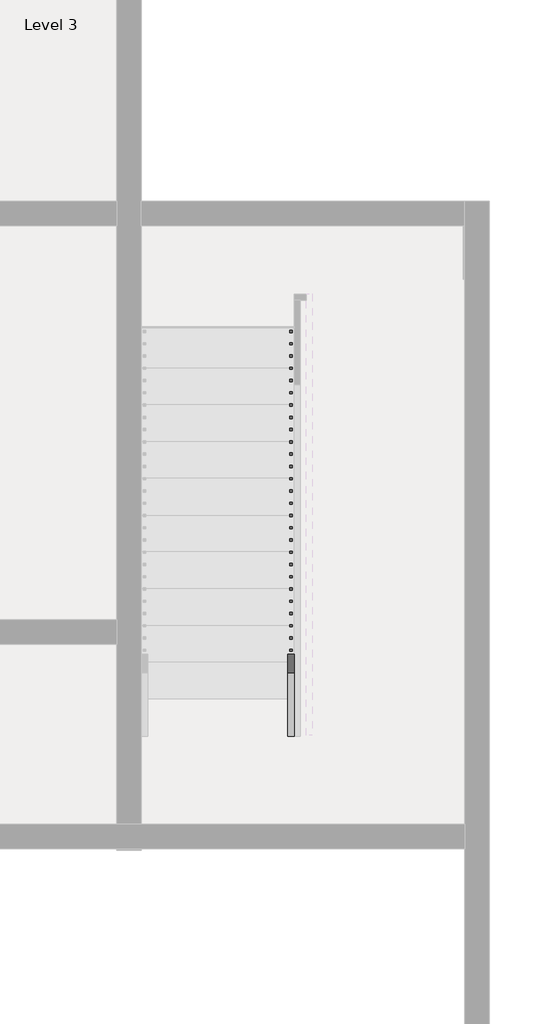
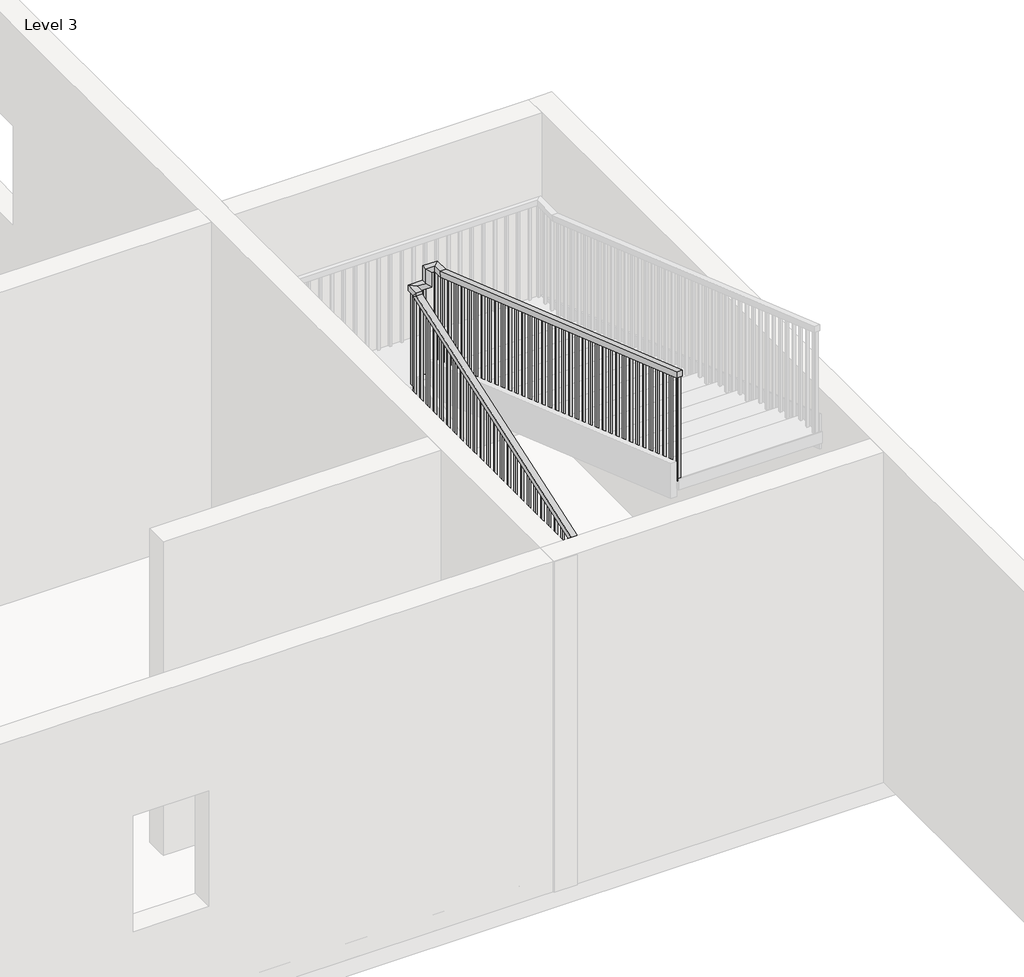
# One storey, part 6 of 14: 1 railing.
"""IFC4 building model written with IfcOpenShell, lengths in millimetres."""

from ifc_helpers import new_model, si_unit, frame, origin, place, context, project, spatial, polyline, outline, extrude, faceted_brep, element, save

model = new_model("IFC4")

# Units and contexts
model_context = context("Model", 3, world=origin())
ifc_project = project(units=[si_unit("LENGTHUNIT", "METRE", prefix="MILLI")], contexts=[model_context])

# Site, building, storey
site = spatial("IfcSite", under=ifc_project)
building = spatial("IfcBuilding", under=site)
storey = spatial("IfcBuildingStorey", under=building, Name="Level 3", Elevation=6096.0)

# Railing
placement = place(None, origin())
element("IfcRailing", 1, ObjectType="Handrail - Rectangular", at=placement, inside=storey, context=model_context, shape_type="SolidModel", body=[
    faceted_brep([(-2644.5381751, -9955.5916506, 7115.9076923), (-2644.5381751, -9955.5916506, 7062.1602476), (-2593.7381751, -9955.5916506, 7062.1602476), (-2593.7381751, -9955.5916506, 7115.9076923), (-2644.5381751, -6367.8416506, 8355.6687908), (-2644.5381751, -6317.0416506, 8319.4754856), (-2593.7381751, -6317.0416506, 8319.4754856), (-2593.7381751, -6367.8416506, 8355.6687908), (-2644.5381751, -6367.8416506, 8382.0), (-2644.5381751, -6317.0416506, 8331.2), (-2593.7381751, -6317.0416506, 8331.2), (-2593.7381751, -6367.8416506, 8382.0), (-2644.5381751, -6240.8416506, 8382.0), (-2644.5381751, -6240.8416506, 8331.2), (-2593.7381751, -6291.6416506, 8331.2), (-2593.7381751, -6291.6416506, 8382.0), (-2517.5381751, -6240.8416506, 8382.0), (-2466.7381751, -6240.8416506, 8331.2), (-2466.7381751, -6291.6416506, 8331.2), (-2517.5381751, -6291.6416506, 8382.0), (-2517.5381751, -6240.8416506, 8513.8846154), (-2466.7381751, -6240.8416506, 8463.0846154), (-2466.7381751, -6291.6416506, 8463.0846154), (-2517.5381751, -6291.6416506, 8513.8846154), (-2390.5381751, -6240.8416506, 8513.8846154), (-2390.5381751, -6240.8416506, 8463.0846154), (-2441.3381751, -6291.6416506, 8463.0846154), (-2441.3381751, -6291.6416506, 8513.8846154), (-2390.5381751, -6367.8416506, 8513.8846154), (-2390.5381751, -6376.3852679, 8463.0846154), (-2441.3381751, -6376.3852679, 8463.0846154), (-2441.3381751, -6367.8416506, 8513.8846154), (-2390.5381751, -9949.2416506, 9753.6), (-2441.3381751, -9949.2416506, 9753.6), (-2441.3381751, -9949.2416506, 9699.842594), (-2390.5381751, -9949.2416506, 9699.842594)], [[[0, 1, 2, 3]], [[1, 0, 4, 5]], [[2, 1, 5, 6]], [[3, 2, 6, 7]], [[0, 3, 7, 4]], [[5, 4, 8, 9]], [[6, 5, 9, 10]], [[7, 6, 10, 11]], [[4, 7, 11, 8]], [[9, 8, 12, 13]], [[10, 9, 13, 14]], [[11, 10, 14, 15]], [[8, 11, 15, 12]], [[13, 12, 16, 17]], [[14, 13, 17, 18]], [[15, 14, 18, 19]], [[12, 15, 19, 16]], [[17, 16, 20, 21]], [[18, 17, 21, 22]], [[19, 18, 22, 23]], [[16, 19, 23, 20]], [[21, 20, 24, 25]], [[22, 21, 25, 26]], [[23, 22, 26, 27]], [[20, 23, 27, 24]], [[25, 24, 28, 29]], [[26, 25, 29, 30]], [[27, 26, 30, 31]], [[24, 27, 31, 28]], [[32, 33, 34, 35]], [[29, 28, 32, 35]], [[30, 29, 35, 34]], [[31, 30, 34, 33]], [[28, 31, 33, 32]]]),
    extrude(outline(polyline([(-9933.3666506, 9694.3474017), (-9914.3166506, 9687.7531709), (-9914.3166506, 8733.6923077), (-9933.3666506, 8733.6923077), (-9933.3666506, 9694.3474017)])), frame((-2425.4631751, 0.0, 0.0), z_axis=(1.0, 0.0, 0.0), x_axis=(0.0, 1.0, 0.0)), (0.0, 0.0, 1.0), 19.05),
    extrude(outline(polyline([(-9831.7666506, 9659.1781709), (-9812.7166506, 9652.5839402), (-9812.7166506, 8733.6923077), (-9831.7666506, 8733.6923077), (-9831.7666506, 9659.1781709)])), frame((-2425.4631751, 0.0, 0.0), z_axis=(1.0, 0.0, 0.0), x_axis=(0.0, 1.0, 0.0)), (0.0, 0.0, 1.0), 19.05),
    extrude(outline(polyline([(-9730.1666506, 9624.0089402), (-9711.1166506, 9617.4147094), (-9711.1166506, 8733.6923077), (-9730.1666506, 8733.6923077), (-9730.1666506, 9624.0089402)])), frame((-2425.4631751, 0.0, 0.0), z_axis=(1.0, 0.0, 0.0), x_axis=(0.0, 1.0, 0.0)), (0.0, 0.0, 1.0), 19.05),
    extrude(outline(polyline([(-9628.5666506, 9588.8397094), (-9609.5166506, 9582.2454786), (-9609.5166506, 8628.1846154), (-9628.5666506, 8628.1846154), (-9628.5666506, 9588.8397094)])), frame((-2425.4631751, 0.0, 0.0), z_axis=(1.0, 0.0, 0.0), x_axis=(0.0, 1.0, 0.0)), (0.0, 0.0, 1.0), 19.05),
    extrude(outline(polyline([(-9526.9666506, 9553.6704786), (-9507.9166506, 9547.0762479), (-9507.9166506, 8628.1846154), (-9526.9666506, 8628.1846154), (-9526.9666506, 9553.6704786)])), frame((-2425.4631751, 0.0, 0.0), z_axis=(1.0, 0.0, 0.0), x_axis=(0.0, 1.0, 0.0)), (0.0, 0.0, 1.0), 19.05),
    extrude(outline(polyline([(-9425.3666506, 9518.5012479), (-9406.3166506, 9511.9070171), (-9406.3166506, 8628.1846154), (-9425.3666506, 8628.1846154), (-9425.3666506, 9518.5012479)])), frame((-2425.4631751, 0.0, 0.0), z_axis=(1.0, 0.0, 0.0), x_axis=(0.0, 1.0, 0.0)), (0.0, 0.0, 1.0), 19.05),
    extrude(outline(polyline([(-9323.7666506, 9483.3320171), (-9304.7166506, 9476.7377863), (-9304.7166506, 8522.6769231), (-9323.7666506, 8522.6769231), (-9323.7666506, 9483.3320171)])), frame((-2425.4631751, 0.0, 0.0), z_axis=(1.0, 0.0, 0.0), x_axis=(0.0, 1.0, 0.0)), (0.0, 0.0, 1.0), 19.05),
    extrude(outline(polyline([(-9222.1666506, 9448.1627863), (-9203.1166506, 9441.5685556), (-9203.1166506, 8522.6769231), (-9222.1666506, 8522.6769231), (-9222.1666506, 9448.1627863)])), frame((-2425.4631751, 0.0, 0.0), z_axis=(1.0, 0.0, 0.0), x_axis=(0.0, 1.0, 0.0)), (0.0, 0.0, 1.0), 19.05),
    extrude(outline(polyline([(-9120.5666506, 9412.9935556), (-9101.5166506, 9406.3993248), (-9101.5166506, 8522.6769231), (-9120.5666506, 8522.6769231), (-9120.5666506, 9412.9935556)])), frame((-2425.4631751, 0.0, 0.0), z_axis=(1.0, 0.0, 0.0), x_axis=(0.0, 1.0, 0.0)), (0.0, 0.0, 1.0), 19.05),
    extrude(outline(polyline([(-9018.9666506, 9377.8243248), (-8999.9166506, 9371.230094), (-8999.9166506, 8417.1692308), (-9018.9666506, 8417.1692308), (-9018.9666506, 9377.8243248)])), frame((-2425.4631751, 0.0, 0.0), z_axis=(1.0, 0.0, 0.0), x_axis=(0.0, 1.0, 0.0)), (0.0, 0.0, 1.0), 19.05),
    extrude(outline(polyline([(-8917.3666506, 9342.655094), (-8898.3166506, 9336.0608632), (-8898.3166506, 8417.1692308), (-8917.3666506, 8417.1692308), (-8917.3666506, 9342.655094)])), frame((-2425.4631751, 0.0, 0.0), z_axis=(1.0, 0.0, 0.0), x_axis=(0.0, 1.0, 0.0)), (0.0, 0.0, 1.0), 19.05),
    extrude(outline(polyline([(-8815.7666506, 9307.4858632), (-8796.7166506, 9300.8916325), (-8796.7166506, 8417.1692308), (-8815.7666506, 8417.1692308), (-8815.7666506, 9307.4858632)])), frame((-2425.4631751, 0.0, 0.0), z_axis=(1.0, 0.0, 0.0), x_axis=(0.0, 1.0, 0.0)), (0.0, 0.0, 1.0), 19.05),
    extrude(outline(polyline([(-8714.1666506, 9272.3166325), (-8695.1166506, 9265.7224017), (-8695.1166506, 8311.6615385), (-8714.1666506, 8311.6615385), (-8714.1666506, 9272.3166325)])), frame((-2425.4631751, 0.0, 0.0), z_axis=(1.0, 0.0, 0.0), x_axis=(0.0, 1.0, 0.0)), (0.0, 0.0, 1.0), 19.05),
    extrude(outline(polyline([(-8612.5666506, 9237.1474017), (-8593.5166506, 9230.5531709), (-8593.5166506, 8311.6615385), (-8612.5666506, 8311.6615385), (-8612.5666506, 9237.1474017)])), frame((-2425.4631751, 0.0, 0.0), z_axis=(1.0, 0.0, 0.0), x_axis=(0.0, 1.0, 0.0)), (0.0, 0.0, 1.0), 19.05),
    extrude(outline(polyline([(-8510.9666506, 9201.9781709), (-8491.9166506, 9195.3839402), (-8491.9166506, 8311.6615385), (-8510.9666506, 8311.6615385), (-8510.9666506, 9201.9781709)])), frame((-2425.4631751, 0.0, 0.0), z_axis=(1.0, 0.0, 0.0), x_axis=(0.0, 1.0, 0.0)), (0.0, 0.0, 1.0), 19.05),
    extrude(outline(polyline([(-8409.3666506, 9166.8089402), (-8390.3166506, 9160.2147094), (-8390.3166506, 8206.1538462), (-8409.3666506, 8206.1538462), (-8409.3666506, 9166.8089402)])), frame((-2425.4631751, 0.0, 0.0), z_axis=(1.0, 0.0, 0.0), x_axis=(0.0, 1.0, 0.0)), (0.0, 0.0, 1.0), 19.05),
    extrude(outline(polyline([(-8307.7666506, 9131.6397094), (-8288.7166506, 9125.0454786), (-8288.7166506, 8206.1538462), (-8307.7666506, 8206.1538462), (-8307.7666506, 9131.6397094)])), frame((-2425.4631751, 0.0, 0.0), z_axis=(1.0, 0.0, 0.0), x_axis=(0.0, 1.0, 0.0)), (0.0, 0.0, 1.0), 19.05),
    extrude(outline(polyline([(-8206.1666506, 9096.4704786), (-8187.1166506, 9089.8762479), (-8187.1166506, 8206.1538462), (-8206.1666506, 8206.1538462), (-8206.1666506, 9096.4704786)])), frame((-2425.4631751, 0.0, 0.0), z_axis=(1.0, 0.0, 0.0), x_axis=(0.0, 1.0, 0.0)), (0.0, 0.0, 1.0), 19.05),
    extrude(outline(polyline([(-8104.5666506, 9061.3012479), (-8085.5166506, 9054.7070171), (-8085.5166506, 8100.6461538), (-8104.5666506, 8100.6461538), (-8104.5666506, 9061.3012479)])), frame((-2425.4631751, 0.0, 0.0), z_axis=(1.0, 0.0, 0.0), x_axis=(0.0, 1.0, 0.0)), (0.0, 0.0, 1.0), 19.05),
    extrude(outline(polyline([(-8002.9666506, 9026.1320171), (-7983.9166506, 9019.5377863), (-7983.9166506, 8100.6461538), (-8002.9666506, 8100.6461538), (-8002.9666506, 9026.1320171)])), frame((-2425.4631751, 0.0, 0.0), z_axis=(1.0, 0.0, 0.0), x_axis=(0.0, 1.0, 0.0)), (0.0, 0.0, 1.0), 19.05),
    extrude(outline(polyline([(-7901.3666506, 8990.9627863), (-7882.3166506, 8984.3685556), (-7882.3166506, 8100.6461538), (-7901.3666506, 8100.6461538), (-7901.3666506, 8990.9627863)])), frame((-2425.4631751, 0.0, 0.0), z_axis=(1.0, 0.0, 0.0), x_axis=(0.0, 1.0, 0.0)), (0.0, 0.0, 1.0), 19.05),
    extrude(outline(polyline([(-7799.7666506, 8955.7935556), (-7780.7166506, 8949.1993248), (-7780.7166506, 7995.1384615), (-7799.7666506, 7995.1384615), (-7799.7666506, 8955.7935556)])), frame((-2425.4631751, 0.0, 0.0), z_axis=(1.0, 0.0, 0.0), x_axis=(0.0, 1.0, 0.0)), (0.0, 0.0, 1.0), 19.05),
    extrude(outline(polyline([(-7698.1666506, 8920.6243248), (-7679.1166506, 8914.030094), (-7679.1166506, 7995.1384615), (-7698.1666506, 7995.1384615), (-7698.1666506, 8920.6243248)])), frame((-2425.4631751, 0.0, 0.0), z_axis=(1.0, 0.0, 0.0), x_axis=(0.0, 1.0, 0.0)), (0.0, 0.0, 1.0), 19.05),
    extrude(outline(polyline([(-7596.5666506, 8885.455094), (-7577.5166506, 8878.8608632), (-7577.5166506, 7995.1384615), (-7596.5666506, 7995.1384615), (-7596.5666506, 8885.455094)])), frame((-2425.4631751, 0.0, 0.0), z_axis=(1.0, 0.0, 0.0), x_axis=(0.0, 1.0, 0.0)), (0.0, 0.0, 1.0), 19.05),
    extrude(outline(polyline([(-7494.9666506, 8850.2858632), (-7475.9166506, 8843.6916325), (-7475.9166506, 7889.6307692), (-7494.9666506, 7889.6307692), (-7494.9666506, 8850.2858632)])), frame((-2425.4631751, 0.0, 0.0), z_axis=(1.0, 0.0, 0.0), x_axis=(0.0, 1.0, 0.0)), (0.0, 0.0, 1.0), 19.05),
    extrude(outline(polyline([(-7393.3666506, 8815.1166325), (-7374.3166506, 8808.5224017), (-7374.3166506, 7889.6307692), (-7393.3666506, 7889.6307692), (-7393.3666506, 8815.1166325)])), frame((-2425.4631751, 0.0, 0.0), z_axis=(1.0, 0.0, 0.0), x_axis=(0.0, 1.0, 0.0)), (0.0, 0.0, 1.0), 19.05),
    extrude(outline(polyline([(-7291.7666506, 8779.9474017), (-7272.7166506, 8773.3531709), (-7272.7166506, 7889.6307692), (-7291.7666506, 7889.6307692), (-7291.7666506, 8779.9474017)])), frame((-2425.4631751, 0.0, 0.0), z_axis=(1.0, 0.0, 0.0), x_axis=(0.0, 1.0, 0.0)), (0.0, 0.0, 1.0), 19.05),
    extrude(outline(polyline([(-7190.1666506, 8744.7781709), (-7171.1166506, 8738.1839402), (-7171.1166506, 7784.1230769), (-7190.1666506, 7784.1230769), (-7190.1666506, 8744.7781709)])), frame((-2425.4631751, 0.0, 0.0), z_axis=(1.0, 0.0, 0.0), x_axis=(0.0, 1.0, 0.0)), (0.0, 0.0, 1.0), 19.05),
    extrude(outline(polyline([(-7088.5666506, 8709.6089402), (-7069.5166506, 8703.0147094), (-7069.5166506, 7784.1230769), (-7088.5666506, 7784.1230769), (-7088.5666506, 8709.6089402)])), frame((-2425.4631751, 0.0, 0.0), z_axis=(1.0, 0.0, 0.0), x_axis=(0.0, 1.0, 0.0)), (0.0, 0.0, 1.0), 19.05),
    extrude(outline(polyline([(-6986.9666506, 8674.4397094), (-6967.9166506, 8667.8454786), (-6967.9166506, 7784.1230769), (-6986.9666506, 7784.1230769), (-6986.9666506, 8674.4397094)])), frame((-2425.4631751, 0.0, 0.0), z_axis=(1.0, 0.0, 0.0), x_axis=(0.0, 1.0, 0.0)), (0.0, 0.0, 1.0), 19.05),
    extrude(outline(polyline([(-6885.3666506, 8639.2704786), (-6866.3166506, 8632.6762479), (-6866.3166506, 7678.6153846), (-6885.3666506, 7678.6153846), (-6885.3666506, 8639.2704786)])), frame((-2425.4631751, 0.0, 0.0), z_axis=(1.0, 0.0, 0.0), x_axis=(0.0, 1.0, 0.0)), (0.0, 0.0, 1.0), 19.05),
    extrude(outline(polyline([(-6783.7666506, 8604.1012479), (-6764.7166506, 8597.5070171), (-6764.7166506, 7678.6153846), (-6783.7666506, 7678.6153846), (-6783.7666506, 8604.1012479)])), frame((-2425.4631751, 0.0, 0.0), z_axis=(1.0, 0.0, 0.0), x_axis=(0.0, 1.0, 0.0)), (0.0, 0.0, 1.0), 19.05),
    extrude(outline(polyline([(-6682.1666506, 8568.9320171), (-6663.1166506, 8562.3377863), (-6663.1166506, 7678.6153846), (-6682.1666506, 7678.6153846), (-6682.1666506, 8568.9320171)])), frame((-2425.4631751, 0.0, 0.0), z_axis=(1.0, 0.0, 0.0), x_axis=(0.0, 1.0, 0.0)), (0.0, 0.0, 1.0), 19.05),
    extrude(outline(polyline([(-6580.5666506, 8533.7627863), (-6561.5166506, 8527.1685556), (-6561.5166506, 7573.1076923), (-6580.5666506, 7573.1076923), (-6580.5666506, 8533.7627863)])), frame((-2425.4631751, 0.0, 0.0), z_axis=(1.0, 0.0, 0.0), x_axis=(0.0, 1.0, 0.0)), (0.0, 0.0, 1.0), 19.05),
    extrude(outline(polyline([(-6478.9666506, 8498.5935556), (-6459.9166506, 8491.9993248), (-6459.9166506, 7573.1076923), (-6478.9666506, 7573.1076923), (-6478.9666506, 8498.5935556)])), frame((-2425.4631751, 0.0, 0.0), z_axis=(1.0, 0.0, 0.0), x_axis=(0.0, 1.0, 0.0)), (0.0, 0.0, 1.0), 19.05),
    extrude(outline(polyline([(-6377.3666506, 8463.4243248), (-6358.3166506, 8456.830094), (-6358.3166506, 7573.1076923), (-6377.3666506, 7573.1076923), (-6377.3666506, 8463.4243248)])), frame((-2425.4631751, 0.0, 0.0), z_axis=(1.0, 0.0, 0.0), x_axis=(0.0, 1.0, 0.0)), (0.0, 0.0, 1.0), 19.05),
    extrude(outline(polyline([(-2527.0631751, -6275.7666506), (-2527.0631751, -6256.7166506), (-2508.0131751, -6256.7166506), (-2508.0131751, -6275.7666506), (-2527.0631751, -6275.7666506)])), frame((0.0, 0.0, 7467.6), z_axis=(0.0, 0.0, 1.0), x_axis=(1.0, 0.0, 0.0)), (0.0, 0.0, 1.0), 863.6),
    extrude(outline(polyline([(-2609.6131751, -6307.5166506), (-2628.6631751, -6307.5166506), (-2628.6631751, -6288.4666506), (-2609.6131751, -6288.4666506), (-2609.6131751, -6307.5166506)])), frame((0.0, 0.0, 7362.0923077), z_axis=(0.0, 0.0, 1.0), x_axis=(1.0, 0.0, 0.0)), (0.0, 0.0, 1.0), 969.1076923),
    extrude(outline(polyline([(-6409.1166506, 8287.6586078), (-6390.0666506, 8294.2414101), (-6390.0666506, 7362.0923077), (-6409.1166506, 7362.0923077), (-6409.1166506, 8287.6586078)])), frame((-2628.6631751, 0.0, 0.0), z_axis=(1.0, 0.0, 0.0), x_axis=(0.0, 1.0, 0.0)), (0.0, 0.0, 1.0), 19.05),
    extrude(outline(polyline([(-6510.7166506, 8252.5503289), (-6491.6666506, 8259.1331312), (-6491.6666506, 7362.0923077), (-6510.7166506, 7362.0923077), (-6510.7166506, 8252.5503289)])), frame((-2628.6631751, 0.0, 0.0), z_axis=(1.0, 0.0, 0.0), x_axis=(0.0, 1.0, 0.0)), (0.0, 0.0, 1.0), 19.05),
    extrude(outline(polyline([(-6612.3166506, 8217.44205), (-6593.2666506, 8224.0248523), (-6593.2666506, 7256.5846154), (-6612.3166506, 7256.5846154), (-6612.3166506, 8217.44205)])), frame((-2628.6631751, 0.0, 0.0), z_axis=(1.0, 0.0, 0.0), x_axis=(0.0, 1.0, 0.0)), (0.0, 0.0, 1.0), 19.05),
    extrude(outline(polyline([(-6713.9166506, 8182.3337711), (-6694.8666506, 8188.9165734), (-6694.8666506, 7256.5846154), (-6713.9166506, 7256.5846154), (-6713.9166506, 8182.3337711)])), frame((-2628.6631751, 0.0, 0.0), z_axis=(1.0, 0.0, 0.0), x_axis=(0.0, 1.0, 0.0)), (0.0, 0.0, 1.0), 19.05),
    extrude(outline(polyline([(-6815.5166506, 8147.2254922), (-6796.4666506, 8153.8082945), (-6796.4666506, 7256.5846154), (-6815.5166506, 7256.5846154), (-6815.5166506, 8147.2254922)])), frame((-2628.6631751, 0.0, 0.0), z_axis=(1.0, 0.0, 0.0), x_axis=(0.0, 1.0, 0.0)), (0.0, 0.0, 1.0), 19.05),
    extrude(outline(polyline([(-6917.1166506, 8112.1172133), (-6898.0666506, 8118.7000156), (-6898.0666506, 7151.0769231), (-6917.1166506, 7151.0769231), (-6917.1166506, 8112.1172133)])), frame((-2628.6631751, 0.0, 0.0), z_axis=(1.0, 0.0, 0.0), x_axis=(0.0, 1.0, 0.0)), (0.0, 0.0, 1.0), 19.05),
    extrude(outline(polyline([(-7018.7166506, 8077.0089344), (-6999.6666506, 8083.5917367), (-6999.6666506, 7151.0769231), (-7018.7166506, 7151.0769231), (-7018.7166506, 8077.0089344)])), frame((-2628.6631751, 0.0, 0.0), z_axis=(1.0, 0.0, 0.0), x_axis=(0.0, 1.0, 0.0)), (0.0, 0.0, 1.0), 19.05),
    extrude(outline(polyline([(-7120.3166506, 8041.9006556), (-7101.2666506, 8048.4834578), (-7101.2666506, 7151.0769231), (-7120.3166506, 7151.0769231), (-7120.3166506, 8041.9006556)])), frame((-2628.6631751, 0.0, 0.0), z_axis=(1.0, 0.0, 0.0), x_axis=(0.0, 1.0, 0.0)), (0.0, 0.0, 1.0), 19.05),
    extrude(outline(polyline([(-7221.9166506, 8006.7923767), (-7202.8666506, 8013.3751789), (-7202.8666506, 7045.5692308), (-7221.9166506, 7045.5692308), (-7221.9166506, 8006.7923767)])), frame((-2628.6631751, 0.0, 0.0), z_axis=(1.0, 0.0, 0.0), x_axis=(0.0, 1.0, 0.0)), (0.0, 0.0, 1.0), 19.05),
    extrude(outline(polyline([(-7323.5166506, 7971.6840978), (-7304.4666506, 7978.2669001), (-7304.4666506, 7045.5692308), (-7323.5166506, 7045.5692308), (-7323.5166506, 7971.6840978)])), frame((-2628.6631751, 0.0, 0.0), z_axis=(1.0, 0.0, 0.0), x_axis=(0.0, 1.0, 0.0)), (0.0, 0.0, 1.0), 19.05),
    extrude(outline(polyline([(-7425.1166506, 7936.5758189), (-7406.0666506, 7943.1586212), (-7406.0666506, 7045.5692308), (-7425.1166506, 7045.5692308), (-7425.1166506, 7936.5758189)])), frame((-2628.6631751, 0.0, 0.0), z_axis=(1.0, 0.0, 0.0), x_axis=(0.0, 1.0, 0.0)), (0.0, 0.0, 1.0), 19.05),
    extrude(outline(polyline([(-7526.7166506, 7901.46754), (-7507.6666506, 7908.0503423), (-7507.6666506, 6940.0615385), (-7526.7166506, 6940.0615385), (-7526.7166506, 7901.46754)])), frame((-2628.6631751, 0.0, 0.0), z_axis=(1.0, 0.0, 0.0), x_axis=(0.0, 1.0, 0.0)), (0.0, 0.0, 1.0), 19.05),
    extrude(outline(polyline([(-7628.3166506, 7866.3592611), (-7609.2666506, 7872.9420634), (-7609.2666506, 6940.0615385), (-7628.3166506, 6940.0615385), (-7628.3166506, 7866.3592611)])), frame((-2628.6631751, 0.0, 0.0), z_axis=(1.0, 0.0, 0.0), x_axis=(0.0, 1.0, 0.0)), (0.0, 0.0, 1.0), 19.05),
    extrude(outline(polyline([(-7729.9166506, 7831.2509822), (-7710.8666506, 7837.8337845), (-7710.8666506, 6940.0615385), (-7729.9166506, 6940.0615385), (-7729.9166506, 7831.2509822)])), frame((-2628.6631751, 0.0, 0.0), z_axis=(1.0, 0.0, 0.0), x_axis=(0.0, 1.0, 0.0)), (0.0, 0.0, 1.0), 19.05),
    extrude(outline(polyline([(-7831.5166506, 7796.1427033), (-7812.4666506, 7802.7255056), (-7812.4666506, 6834.5538462), (-7831.5166506, 6834.5538462), (-7831.5166506, 7796.1427033)])), frame((-2628.6631751, 0.0, 0.0), z_axis=(1.0, 0.0, 0.0), x_axis=(0.0, 1.0, 0.0)), (0.0, 0.0, 1.0), 19.05),
    extrude(outline(polyline([(-7933.1166506, 7761.0344244), (-7914.0666506, 7767.6172267), (-7914.0666506, 6834.5538462), (-7933.1166506, 6834.5538462), (-7933.1166506, 7761.0344244)])), frame((-2628.6631751, 0.0, 0.0), z_axis=(1.0, 0.0, 0.0), x_axis=(0.0, 1.0, 0.0)), (0.0, 0.0, 1.0), 19.05),
    extrude(outline(polyline([(-8034.7166506, 7725.9261455), (-8015.6666506, 7732.5089478), (-8015.6666506, 6834.5538462), (-8034.7166506, 6834.5538462), (-8034.7166506, 7725.9261455)])), frame((-2628.6631751, 0.0, 0.0), z_axis=(1.0, 0.0, 0.0), x_axis=(0.0, 1.0, 0.0)), (0.0, 0.0, 1.0), 19.05),
    extrude(outline(polyline([(-8136.3166506, 7690.8178666), (-8117.2666506, 7697.4006689), (-8117.2666506, 6729.0461538), (-8136.3166506, 6729.0461538), (-8136.3166506, 7690.8178666)])), frame((-2628.6631751, 0.0, 0.0), z_axis=(1.0, 0.0, 0.0), x_axis=(0.0, 1.0, 0.0)), (0.0, 0.0, 1.0), 19.05),
    extrude(outline(polyline([(-8237.9166506, 7655.7095877), (-8218.8666506, 7662.29239), (-8218.8666506, 6729.0461538), (-8237.9166506, 6729.0461538), (-8237.9166506, 7655.7095877)])), frame((-2628.6631751, 0.0, 0.0), z_axis=(1.0, 0.0, 0.0), x_axis=(0.0, 1.0, 0.0)), (0.0, 0.0, 1.0), 19.05),
    extrude(outline(polyline([(-8339.5166506, 7620.6013088), (-8320.4666506, 7627.1841111), (-8320.4666506, 6729.0461538), (-8339.5166506, 6729.0461538), (-8339.5166506, 7620.6013088)])), frame((-2628.6631751, 0.0, 0.0), z_axis=(1.0, 0.0, 0.0), x_axis=(0.0, 1.0, 0.0)), (0.0, 0.0, 1.0), 19.05),
    extrude(outline(polyline([(-8441.1166506, 7585.4930299), (-8422.0666506, 7592.0758322), (-8422.0666506, 6623.5384615), (-8441.1166506, 6623.5384615), (-8441.1166506, 7585.4930299)])), frame((-2628.6631751, 0.0, 0.0), z_axis=(1.0, 0.0, 0.0), x_axis=(0.0, 1.0, 0.0)), (0.0, 0.0, 1.0), 19.05),
    extrude(outline(polyline([(-8542.7166506, 7550.384751), (-8523.6666506, 7556.9675533), (-8523.6666506, 6623.5384615), (-8542.7166506, 6623.5384615), (-8542.7166506, 7550.384751)])), frame((-2628.6631751, 0.0, 0.0), z_axis=(1.0, 0.0, 0.0), x_axis=(0.0, 1.0, 0.0)), (0.0, 0.0, 1.0), 19.05),
    extrude(outline(polyline([(-8644.3166506, 7515.2764721), (-8625.2666506, 7521.8592744), (-8625.2666506, 6623.5384615), (-8644.3166506, 6623.5384615), (-8644.3166506, 7515.2764721)])), frame((-2628.6631751, 0.0, 0.0), z_axis=(1.0, 0.0, 0.0), x_axis=(0.0, 1.0, 0.0)), (0.0, 0.0, 1.0), 19.05),
    extrude(outline(polyline([(-8745.9166506, 7480.1681932), (-8726.8666506, 7486.7509955), (-8726.8666506, 6518.0307692), (-8745.9166506, 6518.0307692), (-8745.9166506, 7480.1681932)])), frame((-2628.6631751, 0.0, 0.0), z_axis=(1.0, 0.0, 0.0), x_axis=(0.0, 1.0, 0.0)), (0.0, 0.0, 1.0), 19.05),
    extrude(outline(polyline([(-8847.5166506, 7445.0599143), (-8828.4666506, 7451.6427166), (-8828.4666506, 6518.0307692), (-8847.5166506, 6518.0307692), (-8847.5166506, 7445.0599143)])), frame((-2628.6631751, 0.0, 0.0), z_axis=(1.0, 0.0, 0.0), x_axis=(0.0, 1.0, 0.0)), (0.0, 0.0, 1.0), 19.05),
    extrude(outline(polyline([(-8949.1166506, 7409.9516354), (-8930.0666506, 7416.5344377), (-8930.0666506, 6518.0307692), (-8949.1166506, 6518.0307692), (-8949.1166506, 7409.9516354)])), frame((-2628.6631751, 0.0, 0.0), z_axis=(1.0, 0.0, 0.0), x_axis=(0.0, 1.0, 0.0)), (0.0, 0.0, 1.0), 19.05),
    extrude(outline(polyline([(-9050.7166506, 7374.8433565), (-9031.6666506, 7381.4261588), (-9031.6666506, 6412.5230769), (-9050.7166506, 6412.5230769), (-9050.7166506, 7374.8433565)])), frame((-2628.6631751, 0.0, 0.0), z_axis=(1.0, 0.0, 0.0), x_axis=(0.0, 1.0, 0.0)), (0.0, 0.0, 1.0), 19.05),
    extrude(outline(polyline([(-9152.3166506, 7339.7350776), (-9133.2666506, 7346.3178799), (-9133.2666506, 6412.5230769), (-9152.3166506, 6412.5230769), (-9152.3166506, 7339.7350776)])), frame((-2628.6631751, 0.0, 0.0), z_axis=(1.0, 0.0, 0.0), x_axis=(0.0, 1.0, 0.0)), (0.0, 0.0, 1.0), 19.05),
    extrude(outline(polyline([(-9253.9166506, 7304.6267987), (-9234.8666506, 7311.209601), (-9234.8666506, 6412.5230769), (-9253.9166506, 6412.5230769), (-9253.9166506, 7304.6267987)])), frame((-2628.6631751, 0.0, 0.0), z_axis=(1.0, 0.0, 0.0), x_axis=(0.0, 1.0, 0.0)), (0.0, 0.0, 1.0), 19.05),
    extrude(outline(polyline([(-9355.5166506, 7269.5185198), (-9336.4666506, 7276.1013221), (-9336.4666506, 6307.0153846), (-9355.5166506, 6307.0153846), (-9355.5166506, 7269.5185198)])), frame((-2628.6631751, 0.0, 0.0), z_axis=(1.0, 0.0, 0.0), x_axis=(0.0, 1.0, 0.0)), (0.0, 0.0, 1.0), 19.05),
    extrude(outline(polyline([(-9457.1166506, 7234.4102409), (-9438.0666506, 7240.9930432), (-9438.0666506, 6307.0153846), (-9457.1166506, 6307.0153846), (-9457.1166506, 7234.4102409)])), frame((-2628.6631751, 0.0, 0.0), z_axis=(1.0, 0.0, 0.0), x_axis=(0.0, 1.0, 0.0)), (0.0, 0.0, 1.0), 19.05),
    extrude(outline(polyline([(-9558.7166506, 7199.301962), (-9539.6666506, 7205.8847643), (-9539.6666506, 6307.0153846), (-9558.7166506, 6307.0153846), (-9558.7166506, 7199.301962)])), frame((-2628.6631751, 0.0, 0.0), z_axis=(1.0, 0.0, 0.0), x_axis=(0.0, 1.0, 0.0)), (0.0, 0.0, 1.0), 19.05),
    extrude(outline(polyline([(-9660.3166506, 7164.1936831), (-9641.2666506, 7170.7764854), (-9641.2666506, 6201.5076923), (-9660.3166506, 6201.5076923), (-9660.3166506, 7164.1936831)])), frame((-2628.6631751, 0.0, 0.0), z_axis=(1.0, 0.0, 0.0), x_axis=(0.0, 1.0, 0.0)), (0.0, 0.0, 1.0), 19.05),
    extrude(outline(polyline([(-9761.9166506, 7129.0854043), (-9742.8666506, 7135.6682065), (-9742.8666506, 6201.5076923), (-9761.9166506, 6201.5076923), (-9761.9166506, 7129.0854043)])), frame((-2628.6631751, 0.0, 0.0), z_axis=(1.0, 0.0, 0.0), x_axis=(0.0, 1.0, 0.0)), (0.0, 0.0, 1.0), 19.05),
    extrude(outline(polyline([(-9863.5166506, 7093.9771254), (-9844.4666506, 7100.5599277), (-9844.4666506, 6201.5076923), (-9863.5166506, 6201.5076923), (-9863.5166506, 7093.9771254)])), frame((-2628.6631751, 0.0, 0.0), z_axis=(1.0, 0.0, 0.0), x_axis=(0.0, 1.0, 0.0)), (0.0, 0.0, 1.0), 19.05),
    extrude(outline(polyline([(-2425.4631751, -6275.7666506), (-2425.4631751, -6256.7166506), (-2406.4131751, -6256.7166506), (-2406.4131751, -6275.7666506), (-2425.4631751, -6275.7666506)])), frame((0.0, 0.0, 7467.6), z_axis=(0.0, 0.0, 1.0), x_axis=(1.0, 0.0, 0.0)), (0.0, 0.0, 1.0), 995.4846154),
    extrude(outline(polyline([(-2609.6131751, -6275.7666506), (-2628.6631751, -6275.7666506), (-2628.6631751, -6256.7166506), (-2609.6131751, -6256.7166506), (-2609.6131751, -6275.7666506)])), frame((0.0, 0.0, 7467.6), z_axis=(0.0, 0.0, 1.0), x_axis=(1.0, 0.0, 0.0)), (0.0, 0.0, 1.0), 863.6),
    extrude(outline(polyline([(-9949.2416506, 9699.842594), (-9930.1916506, 9693.2483632), (-9930.1916506, 8733.6923077), (-9949.2416506, 8733.6923077), (-9949.2416506, 9699.842594)])), frame((-2425.4631751, 0.0, 0.0), z_axis=(1.0, 0.0, 0.0), x_axis=(0.0, 1.0, 0.0)), (0.0, 0.0, 1.0), 19.05),
    extrude(outline(polyline([(-9955.5916506, 7062.1602476), (-9936.5416506, 7068.7430499), (-9936.5416506, 6201.5076923), (-9955.5916506, 6201.5076923), (-9955.5916506, 7062.1602476)])), frame((-2628.6631751, 0.0, 0.0), z_axis=(1.0, 0.0, 0.0), x_axis=(0.0, 1.0, 0.0)), (0.0, 0.0, 1.0), 19.05),
])

save(model, "model.ifc")

# Revit data of these elements
# Type "Handrail - Rectangular"
#   Assembly Code = "C2010400"
#   built-in parameter 1008612 = 0.0416667 (stored number, unit not read)
#   built-in parameter 1008611 = 0.0416667 (stored number, unit not read)
#   built-in parameter 1008609 = 0.333333 (stored number, unit not read)
#   built-in parameter 1008604 = 0.166667 (stored number, unit not read)
#   built-in parameter 1008603 = 0.166667 (stored number, unit not read)
#   Railing Height = 3' - 0"
#   built-in parameter 1008630 = 2
#   built-in parameter 1008610 = 2
#   built-in parameter 1008618 = Baluster - Square : 3/4"
# Element 1 (IfcRailing, "Handrail - Rectangular")
#   Phase Created = New Construction
